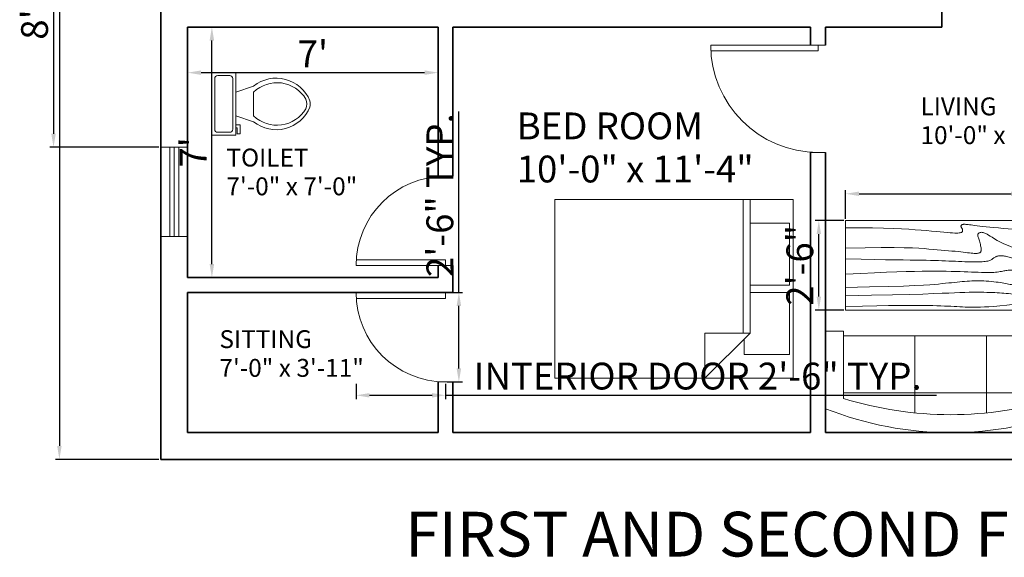
# Model space of a CAD drawing. Units: inches. Extents: x 3087 to 8148, y 1377 to 3709.
# Tile 1 of 6: x 3112 to 3443, y 1381 to 1561. Entities that reach past the tile are written whole.
import ezdxf

# ---------------------------------------------------------------- set-up
doc = ezdxf.new("R2010")
doc.units = ezdxf.units.IN
for name, color, linetype, lineweight, true_color in [('A-ANNO-DIMS', 244, 'Continuous', 18, 0x991b1e), ('A-ANNO-TEXT', 244, 'Continuous', 25, 0x991b1e), ('A-AREA-IDEN', 244, 'Continuous', 18, 0x991b1e), ('A-DOOR', 146, 'Continuous', 18, 0x105689), ('A-GLAZ', 146, 'Continuous', 18, 0x105689), ('A-WALL', 241, 'Continuous', 35, 0xf7abae)]:
    doc.layers.add(name, color=color, linetype=linetype, lineweight=lineweight, true_color=true_color)
doc.layers.add('A-FLOR-FIXT', color=9, linetype='Continuous', lineweight=18)
doc.layers.add('A-FURN', color=8, linetype='Continuous', lineweight=18)
doc.styles.get("Standard").update_dxf_attribs({"font": 'arial.ttf'})
doc.dimstyles.new('ISO-25', dxfattribs={"dimtxt": 9, "dimasz": 4.5, "dimexe": 1.25, "dimexo": 0.625, "dimtad": 1, "dimdec": 0, "dimlunit": 3, "dimtxsty": 'Standard', "dimcen": 2.5, "dimadec": 0, "dimazin": 0, "dimtfac": 1, "dimtdec": 0, "dimtmove": 0, "dimatfit": 3, "dimfxl": 1, "dimarcsym": 0})

# ---------------------------------------------------------------- blocks, each defined once
blk = doc.blocks.new('Bed - Queen')
for p, q in [((0, -80.00003), (0, 0)), ((0, 0), (59.99999, 0)), ((59.99999, 0), (59.99999, -80.00003)), ((7.99999, -1.2), (28.79998, -1.2)), ((7.99999, -14.4), (7.99999, -1.2)), ((28.79998, -1.2), (28.79998, -14.4)), ((31.19999, -1.2), (51.99999, -1.2)), ((31.19999, -14.4), (31.19999, -1.2)), ((51.99999, -1.2), (51.99999, -16.4)), ((0, -14.4), (44.8, -14.4)), ((59.99999, -29.6), (44.8, -14.4)), ((44.8, -14.4), (44.8, -29.6)), ((51.99999, -16.4), (46.79936, -16.4)), ((44.8, -16.8), (0, -16.8)), ((44.8, -29.6), (59.99999, -29.6)), ((59.99999, -80.00003), (0, -80.00003))]:
    blk.add_line(p, q)
blk = doc.blocks.new('Table - Rectangular Woodgrain 60 x 30 in.')
for p, q in [((0, 0), (0, -30)), ((60, 0), (0, 0)), ((60, -30), (60, 0)), ((0, -30), (60, -30))]:
    blk.add_line(p, q)
for points in [[(0, -2.4), (4.8155, -2.418), (9.0302, -2.4688), (12.709, -2.5477), (15.9167, -2.65), (18.7181, -2.7711), (21.1781, -2.9063), (23.3616, -3.0508), (25.3333, -3.2), (27.1477, -3.3495), (28.8172, -3.4958), (30.3437, -3.636), (31.7291, -3.7667), (32.9756, -3.8849), (34.0849, -3.9875), (35.059, -4.0714), (35.9, -4.1334), (36.6114, -4.1711), (37.2041, -4.1854), (37.6906, -4.1779), (38.0833, -4.15), (38.3948, -4.1034), (38.6375, -4.0396), (38.8239, -3.9602), (38.9666, -3.8667), (39.0764, -3.7608), (39.1573, -3.6448), (39.2116, -3.521), (39.2416, -3.3917), (39.2498, -3.2593), (39.2385, -3.1261), (39.21, -2.9944), (39.1666, -2.8667), (39.111, -2.7447), (39.0468, -2.6281), (38.978, -2.5163), (38.9083, -2.4083), (38.8418, -2.3035), (38.7823, -2.201), (38.7337, -2.1001), (38.7, -2), (38.6844, -1.9003), (38.6875, -1.8021), (38.7094, -1.707), (38.75, -1.6167), (38.8094, -1.5326), (38.8875, -1.4563), (38.9844, -1.3893), (39.1, -1.3333), (39.2351, -1.2896), (39.3937, -1.2583), (39.5804, -1.2396), (39.8, -1.2333), (40.057, -1.2396), (40.3562, -1.2583), (40.7023, -1.2896), (41.1, -1.3333), (41.5547, -1.3895), (42.0755, -1.4573), (42.6721, -1.5361), (43.3542, -1.625), (44.1316, -1.7233), (45.014, -1.8302), (46.0114, -1.9449), (47.1333, -2.0667), (48.3862, -2.1947), (49.7625, -2.3281), (51.2513, -2.4663), (52.8416, -2.6083), (54.5226, -2.7535), (56.2833, -2.9011), (58.1127, -3.0501), (60, -3.2)], [(0, -9.2), (6.5759, -9.0858), (11.9385, -9.0365), (16.2527, -9.0418), (19.6833, -9.0917), (22.3952, -9.1759), (24.5531, -9.2844), (26.322, -9.4069), (27.8666, -9.5333), (29.3241, -9.6553), (30.7203, -9.7719), (32.0532, -9.8837), (33.3208, -9.9917), (34.5213, -10.0965), (35.6526, -10.199), (36.7128, -10.2999), (37.7, -10.4), (38.6129, -10.4996), (39.4531, -10.5969), (40.223, -10.6895), (40.925, -10.775), (41.5613, -10.8512), (42.1344, -10.9156), (42.6465, -10.966), (43.1, -11), (43.4976, -11.0158), (43.8437, -11.0136), (44.143, -10.9942), (44.4, -10.9583), (44.6195, -10.9069), (44.8062, -10.8406), (44.9648, -10.7603), (45.1, -10.6667), (45.2155, -10.5598), (45.3114, -10.4365), (45.3871, -10.2929), (45.4416, -10.125), (45.4743, -9.929), (45.4844, -9.7011), (45.4709, -9.4371), (45.4333, -9.1333), (45.3716, -8.7883), (45.2896, -8.4104), (45.1919, -8.0107), (45.0833, -7.6), (44.9685, -7.1893), (44.8521, -6.7896), (44.7388, -6.4117), (44.6333, -6.0667), (44.54, -5.7628), (44.4614, -5.4979), (44.4001, -5.2675), (44.3583, -5.0667), (44.3384, -4.8909), (44.3427, -4.7354), (44.3736, -4.5956), (44.4333, -4.4667), (44.5236, -4.3453), (44.6427, -4.2333), (44.7884, -4.1339), (44.9583, -4.05), (45.1501, -3.9849), (45.3614, -3.9417), (45.59, -3.9234), (45.8333, -3.9333), (46.0915, -3.9749), (46.3734, -4.0531), (46.6906, -4.1736), (47.0542, -4.3417), (47.4756, -4.5629), (47.9661, -4.8427), (48.5372, -5.1866), (49.2, -5.6), (49.9676, -6.0844), (50.8594, -6.625), (51.8965, -7.2031), (53.1, -7.8), (54.491, -8.3969), (56.0906, -8.975), (57.9199, -9.5156), (60, -10)], [(0, -12.8), (5.1847, -12.9322), (9.6213, -13.0323), (13.3963, -13.1059), (16.5958, -13.1583), (19.3063, -13.1952), (21.614, -13.2219), (23.6054, -13.2439), (25.3666, -13.2667), (26.9728, -13.2947), (28.4531, -13.3281), (29.8256, -13.3663), (31.1083, -13.4083), (32.3191, -13.4535), (33.476, -13.501), (34.597, -13.5501), (35.7, -13.6), (36.7984, -13.6497), (37.8875, -13.6979), (38.9578, -13.743), (40, -13.7833), (41.0047, -13.8174), (41.9625, -13.8438), (42.864, -13.8607), (43.7, -13.8667), (44.4631, -13.8604), (45.1552, -13.8417), (45.7801, -13.8104), (46.3416, -13.7667), (46.8439, -13.7104), (47.2906, -13.6417), (47.6858, -13.5604), (48.0333, -13.4667), (48.3375, -13.3608), (48.6042, -13.2448), (48.8396, -13.121), (49.05, -12.9917), (49.2417, -12.8593), (49.4208, -12.7261), (49.5937, -12.5944), (49.7667, -12.4667), (49.9452, -12.3451), (50.1323, -12.2313), (50.3303, -12.1268), (50.5416, -12.0333), (50.7686, -11.9524), (51.0135, -11.8854), (51.2788, -11.8341), (51.5666, -11.8), (51.8785, -11.7843), (52.2116, -11.7865), (52.562, -11.8059), (52.926, -11.8417), (53.2998, -11.8931), (53.6795, -11.9594), (54.0614, -12.0397), (54.4416, -12.1333), (54.8223, -12.2401), (55.2293, -12.3625), (55.6942, -12.5037), (56.2489, -12.6667), (56.9251, -12.8547), (57.7545, -13.0708), (58.7689, -13.3182), (60, -13.6)], [(0, -18), (5.124, -17.7273), (9.6609, -17.5057), (13.6705, -17.3303), (17.2125, -17.1958), (20.3467, -17.0973), (23.1328, -17.0297), (25.6307, -16.9878), (27.9, -16.9667), (29.9928, -16.9617), (31.9302, -16.9703), (33.7254, -16.9907), (35.3917, -17.0208), (36.9423, -17.0588), (38.3906, -17.1026), (39.7499, -17.1503), (41.0333, -17.2), (42.2519, -17.2496), (43.4073, -17.2969), (44.4986, -17.3395), (45.525, -17.375), (46.4858, -17.4012), (47.3802, -17.4156), (48.2074, -17.416), (48.9667, -17.4), (49.6583, -17.3662), (50.2872, -17.3167), (50.8595, -17.2547), (51.3812, -17.1833), (51.8584, -17.1057), (52.2971, -17.025), (52.7034, -16.9443), (53.0833, -16.8667), (53.443, -16.7951), (53.789, -16.7313), (54.128, -16.6768), (54.4666, -16.6334), (54.8115, -16.6024), (55.1693, -16.5854), (55.5465, -16.5841), (55.95, -16.6), (56.3828, -16.6337), (56.8346, -16.6823), (57.2915, -16.7418), (57.7396, -16.8084), (58.165, -16.878), (58.5539, -16.9469), (58.8924, -17.0111), (59.1666, -17.0667), (59.3679, -17.1107), (59.5078, -17.1438), (59.6032, -17.1675), (59.6708, -17.1833), (59.7275, -17.193), (59.7901, -17.1979), (59.8753, -17.1998), (60, -17.2)], [(0, -22.4), (8.0098, -22.2501), (14.4094, -22.1011), (19.4168, -21.9535), (23.25, -21.8083), (26.1269, -21.6663), (28.2656, -21.5281), (29.884, -21.3947), (31.2, -21.2667), (32.3967, -21.1448), (33.5172, -21.0292), (34.5697, -20.9198), (35.5625, -20.8167), (36.5037, -20.7198), (37.4015, -20.6292), (38.2642, -20.5448), (39.1, -20.4667), (39.9164, -20.3951), (40.7187, -20.3313), (41.5117, -20.2768), (42.3, -20.2333), (43.0883, -20.2024), (43.8812, -20.1854), (44.6836, -20.1841), (45.5, -20.2), (46.3328, -20.234), (47.1747, -20.2844), (48.0163, -20.3488), (48.8479, -20.425), (49.66, -20.5106), (50.4429, -20.6031), (51.1872, -20.7004), (51.8833, -20.8), (52.5246, -20.8999), (53.1166, -20.9995), (53.6681, -21.0983), (54.1875, -21.1958), (54.6834, -21.2919), (55.1646, -21.3859), (55.6394, -21.4777), (56.1167, -21.5667), (56.6028, -21.6515), (57.0961, -21.7266), (57.5929, -21.7852), (58.0896, -21.8208), (58.5823, -21.8268), (59.0674, -21.7964), (59.5412, -21.723), (60, -21.6)], [(0, -25.2), (8.6355, -25.0504), (15.7026, -24.9031), (21.4049, -24.7606), (25.9458, -24.625), (29.529, -24.4988), (32.3578, -24.3844), (34.6359, -24.284), (36.5667, -24.2), (38.3213, -24.1341), (39.9417, -24.0854), (41.437, -24.0523), (42.8167, -24.0333), (44.0901, -24.0268), (45.2667, -24.0313), (46.3557, -24.0451), (47.3667, -24.0667), (48.309, -24.0947), (49.1928, -24.1287), (50.0284, -24.168), (50.826, -24.2125), (51.5959, -24.2617), (52.3483, -24.3151), (53.0935, -24.3725), (53.8417, -24.4334), (54.6009, -24.497), (55.3699, -24.561), (56.1454, -24.6226), (56.9239, -24.6792), (57.7021, -24.7279), (58.4764, -24.7662), (59.2435, -24.7911), (60, -24.8)], [(0, -28.8), (5.6867, -28.6681), (10.45, -28.5698), (14.407, -28.5012), (17.675, -28.4584), (20.3711, -28.4374), (22.6125, -28.4344), (24.5164, -28.4455), (26.2, -28.4667), (27.762, -28.4947), (29.2276, -28.5281), (30.6033, -28.5663), (31.8958, -28.6084), (33.1118, -28.6535), (34.2578, -28.7011), (35.3405, -28.7501), (36.3666, -28.8), (37.3443, -28.8497), (38.288, -28.8974), (39.2137, -28.9412), (40.1375, -28.9792), (41.0753, -29.0093), (42.0432, -29.0297), (43.0572, -29.0384), (44.1333, -29.0333), (45.2936, -29.0114), (46.5843, -28.9641), (48.0579, -28.8816), (49.7666, -28.7542), (51.7629, -28.5721), (54.0989, -28.3255), (56.8272, -28.0048), (60, -27.6)]]:
    blk.add_lwpolyline(points)
blk = doc.blocks.new('Toilet - top')
for p, q in [((9.5, -6), (9.5, -2)), ((-10, -8.5), (-8, -8.5)), ((-10, -9.5), (-10, -8.5)), ((-7, -9.5), (-10, -9.5)), ((-8, -8.5), (-8, -8)), ((-7, -8), (-7, -9.5)), ((-4, -8), (-6, -14)), ((4, -8), (6, -14)), ((4, -14), (-4, -14))]:
    blk.add_line(p, q)
blk.add_lwpolyline([(10.5, -8), (10.5, 0), (-10.5, 0), (-10.5, -8)], close=True)
for points in [[(-9.5, -2), (-9.5, -6)], [(8.5, -1), (-8.5, -1)], [(-8.5, -7), (8.5, -7)]]:
    blk.add_lwpolyline(points)
for centre, radius, start, end in [((-8.62, -1.88), 0.884, 81.8699, 188.1301), ((8.62, -1.88), 0.884, 351.8699, 98.1301), ((-8.62, -6.12), 0.884, 171.8699, 278.1301), ((8.62, -6.12), 0.884, 261.8699, 8.1301), ((3.52, -21.58), 12.17, 141.4691, 247.9714), ((4.2, -21.82), 11.33, 136.3677, 238.9468), ((-3.52, -21.58), 12.17, 292.0284, 38.5307), ((-4.2, -21.82), 11.33, 301.053, 43.6321), ((0, -27.88), 4, 245.7318, 294.2682), ((0, -29), 4, 254.8605, 285.1395)]:
    blk.add_arc(centre, radius, start, end)
blk = doc.blocks.new('Sofa - Roundback 7 ft.')
for p, q in [((-12.00002, -32.4421), (-12.00003, -6.5971)), ((11.99997, -32.4421), (11.99998, -6.5971)), ((-36.000027, -34), (-36.000027, -11.4696)), ((35.99998, -34), (35.99998, -11.4696)), ((-35.999844, -13.3819), (35.9998, -13.3819)), ((-36.000027, -32.4421), (35.99998, -32.4421))]:
    blk.add_line(p, q)
for points in [[(-36.000027, -34), (-42.000027, -34), (-42.000027, -8)], [(41.99998, -8), (41.99998, -34), (35.99998, -34)]]:
    blk.add_lwpolyline(points)
for centre, radius, start, end in [((0, -114.25), 114.25, 68.43141, 111.5686), ((-0.00001, -127.1968), 121.1968, 72.72033, 107.2797)]:
    blk.add_arc(centre, radius, start, end)
blk = doc.blocks.new('*D15')
at = {"layer": 'A-ANNO-DIMS', "color": 0, "lineweight": -2, "transparency": 16777216}
for p, q in [((3210.19, 1558.96), (3175.7, 1558.96)), ((3176.95, 1479.46), (3176.95, 1554.46)), ((3201.15, 1474.96), (3175.7, 1474.96))]:
    blk.add_line(p, q, dxfattribs=at)
at = {"layer": 'A-ANNO-DIMS', "color": 0, "transparency": 16777216}
for points in [[(3176.2, 1554.46), (3177.7, 1554.46), (3176.95, 1558.96)], [(3176.2, 1479.46), (3177.7, 1479.46), (3176.95, 1474.96)]]:
    blk.add_solid(points, dxfattribs=at)
at = {"layer": 'Defpoints', "color": 0, "transparency": 16777216}
for p in [(3176.95, 1558.96), (3210.82, 1558.96), (3201.77, 1474.96)]:
    blk.add_point(p, dxfattribs=at)
at = {"layer": 'A-ANNO-DIMS', "color": 0, "transparency": 16777216, "insert": (3171.82, 1516.96), "char_height": 9, "attachment_point": 5, "rotation": 90}
blk.add_mtext("7'", dxfattribs=at)
blk = doc.blocks.new('*D16')
at = {"layer": 'A-ANNO-DIMS', "color": 0, "lineweight": -2, "transparency": 16777216}
for p, q in [((3168.82, 1544.33), (3168.82, 1544.95)), ((3173.32, 1543.7), (3248.32, 1543.7)), ((3252.82, 1544.33), (3252.82, 1544.95))]:
    blk.add_line(p, q, dxfattribs=at)
at = {"layer": 'A-ANNO-DIMS', "color": 0, "transparency": 16777216}
for points in [[(3173.32, 1544.45), (3173.32, 1542.95), (3168.82, 1543.7)], [(3248.32, 1544.45), (3248.32, 1542.95), (3252.82, 1543.7)]]:
    blk.add_solid(points, dxfattribs=at)
at = {"layer": 'Defpoints', "color": 0, "transparency": 16777216}
for p in [(3168.82, 1543.7), (3252.82, 1543.7), (3252.82, 1543.7)]:
    blk.add_point(p, dxfattribs=at)
at = {"layer": 'A-ANNO-DIMS', "color": 0, "transparency": 16777216, "insert": (3210.82, 1548.83), "char_height": 9, "attachment_point": 5}
blk.add_mtext("7'", dxfattribs=at)
blk = doc.blocks.new('*D18')
at = {"layer": 'A-ANNO-DIMS', "color": 0, "lineweight": -2, "transparency": 16777216}
for p, q in [((3159.19, 2073.96), (3124.53, 2073.96)), ((3125.78, 2069.46), (3125.78, 1418.46)), ((3159.19, 1413.96), (3124.53, 1413.96))]:
    blk.add_line(p, q, dxfattribs=at)
at = {"layer": 'A-ANNO-DIMS', "color": 0, "transparency": 16777216}
for points in [[(3125.03, 2069.46), (3126.53, 2069.46), (3125.78, 2073.96)], [(3125.03, 1418.46), (3126.53, 1418.46), (3125.78, 1413.96)]]:
    blk.add_solid(points, dxfattribs=at)
at = {"layer": 'Defpoints', "color": 0, "transparency": 16777216}
for p in [(3159.82, 2073.96), (3125.78, 1413.96), (3159.82, 1413.96)]:
    blk.add_point(p, dxfattribs=at)
at = {"layer": 'A-ANNO-DIMS', "color": 0, "transparency": 16777216, "insert": (3120.58, 1743.96), "char_height": 9, "attachment_point": 5, "rotation": 90}
blk.add_mtext("55'", dxfattribs=at)
blk = doc.blocks.new('DOOR-SINGLE-30IN')
for p, q in [((0, 30), (30, 30)), ((30, 30), (30, 28)), ((0, 28), (30, 28))]:
    blk.add_line(p, q)
blk.add_arc((30, 30), 30, 180, 270)
blk = doc.blocks.new('DOOR-SINGLE-36IN')
for p, q in [((0, 2), (36, 2)), ((36, 0), (36, 2)), ((0, 0), (36, 0))]:
    blk.add_line(p, q)
blk.add_arc((36, 0), 36, 90, 180)
blk = doc.blocks.new('WINDOW-30IN')
for p, q in [((0, 0), (0, 30)), ((9, 30), (0, 30)), ((3, 30), (3, 0)), ((4.5, 30), (4.5, 0)), ((6, 30), (6, 0)), ((9, 30), (9, 0)), ((9, 0), (0, 0))]:
    blk.add_line(p, q)
blk = doc.blocks.new('*D27')
at = {"layer": 'A-ANNO-DIMS', "color": 0, "lineweight": -2, "transparency": 16777216}
for p, q in [((3225.32, 1439.34), (3225.32, 1434.21)), ((3255.32, 1439.34), (3255.32, 1434.21)), ((3229.82, 1435.46), (3250.82, 1435.46)), ((3255.32, 1435.46), (3420.05, 1435.46))]:
    blk.add_line(p, q, dxfattribs=at)
at = {"layer": 'A-ANNO-DIMS', "color": 0, "transparency": 16777216}
for points in [[(3229.82, 1436.21), (3229.82, 1434.71), (3225.32, 1435.46)], [(3250.82, 1436.21), (3250.82, 1434.71), (3255.32, 1435.46)]]:
    blk.add_solid(points, dxfattribs=at)
at = {"layer": 'Defpoints', "color": 0, "transparency": 16777216}
for p in [(3225.32, 1439.96), (3255.32, 1439.96), (3255.32, 1435.46)]:
    blk.add_point(p, dxfattribs=at)
at = {"layer": 'A-ANNO-DIMS', "color": 0, "transparency": 16777216, "insert": (3339.94, 1440.74), "char_height": 9, "attachment_point": 5}
blk.add_mtext('INTERIOR DOOR 2\'-6" TYP.', dxfattribs=at)
blk = doc.blocks.new('*D28')
at = {"layer": 'A-ANNO-DIMS', "color": 0, "lineweight": -2, "transparency": 16777216}
for p, q in [((3259.82, 1469.96), (3259.82, 1530.72)), ((3255.94, 1469.96), (3261.07, 1469.96)), ((3259.82, 1444.46), (3259.82, 1465.46)), ((3255.94, 1439.96), (3261.07, 1439.96))]:
    blk.add_line(p, q, dxfattribs=at)
at = {"layer": 'A-ANNO-DIMS', "color": 0, "transparency": 16777216}
for points in [[(3259.07, 1465.46), (3260.57, 1465.46), (3259.82, 1469.96)], [(3259.07, 1444.46), (3260.57, 1444.46), (3259.82, 1439.96)]]:
    blk.add_solid(points, dxfattribs=at)
at = {"layer": 'Defpoints', "color": 0, "transparency": 16777216}
for p in [(3255.32, 1469.96), (3259.82, 1469.96), (3255.32, 1439.96)]:
    blk.add_point(p, dxfattribs=at)
at = {"layer": 'A-ANNO-DIMS', "color": 0, "transparency": 16777216, "insert": (3254.6, 1502.59), "char_height": 9, "attachment_point": 5, "rotation": 90}
blk.add_mtext('2\'-6" TYP.', dxfattribs=at)
blk = doc.blocks.new('*D51')
at = {"layer": 'A-ANNO-DIMS', "color": 0, "lineweight": -2, "transparency": 16777216}
for p, q in [((3389.59, 1494.68), (3389.59, 1504.31)), ((3449.59, 1494.68), (3449.59, 1504.31)), ((3394.09, 1503.06), (3445.09, 1503.06)), ((3449.59, 1503.06), (3522.82, 1503.06))]:
    blk.add_line(p, q, dxfattribs=at)
at = {"layer": 'A-ANNO-DIMS', "color": 0, "transparency": 16777216}
for points in [[(3394.09, 1503.81), (3394.09, 1502.31), (3389.59, 1503.06)], [(3445.09, 1503.81), (3445.09, 1502.31), (3449.59, 1503.06)]]:
    blk.add_solid(points, dxfattribs=at)
at = {"layer": 'Defpoints', "color": 0, "transparency": 16777216}
for p in [(3449.59, 1503.06), (3389.59, 1494.06), (3449.59, 1494.06)]:
    blk.add_point(p, dxfattribs=at)
at = {"layer": 'A-ANNO-DIMS', "color": 0, "transparency": 16777216, "insert": (3488.45, 1508.28), "char_height": 9, "attachment_point": 5}
blk.add_mtext('TABLE 5\'-0"', dxfattribs=at)
blk = doc.blocks.new('*D52')
at = {"layer": 'A-ANNO-DIMS', "color": 0, "lineweight": -2, "transparency": 16777216}
for p, q in [((3388.97, 1494.06), (3379.34, 1494.06)), ((3380.59, 1468.56), (3380.59, 1489.56)), ((3388.97, 1464.06), (3379.34, 1464.06))]:
    blk.add_line(p, q, dxfattribs=at)
at = {"layer": 'A-ANNO-DIMS', "color": 0, "transparency": 16777216}
for points in [[(3379.84, 1489.56), (3381.34, 1489.56), (3380.59, 1494.06)], [(3379.84, 1468.56), (3381.34, 1468.56), (3380.59, 1464.06)]]:
    blk.add_solid(points, dxfattribs=at)
at = {"layer": 'Defpoints', "color": 0, "transparency": 16777216}
for p in [(3380.59, 1494.06), (3389.59, 1494.06), (3389.59, 1464.06)]:
    blk.add_point(p, dxfattribs=at)
at = {"layer": 'A-ANNO-DIMS', "color": 0, "transparency": 16777216, "insert": (3375.37, 1479.06), "char_height": 9, "attachment_point": 5, "rotation": 90}
blk.add_mtext('2\'-6"', dxfattribs=at)
blk = doc.blocks.new('*D64')
at = {"layer": 'A-ANNO-DIMS', "color": 0, "lineweight": -2, "transparency": 16777216}
for p, q in [((3159.19, 1624.74), (3122.57, 1624.74)), ((3123.82, 1620.24), (3123.82, 1523.18)), ((3159.19, 1518.68), (3122.57, 1518.68))]:
    blk.add_line(p, q, dxfattribs=at)
at = {"layer": 'A-ANNO-DIMS', "color": 0, "transparency": 16777216}
for points in [[(3123.07, 1620.24), (3124.57, 1620.24), (3123.82, 1624.74)], [(3123.07, 1523.18), (3124.57, 1523.18), (3123.82, 1518.68)]]:
    blk.add_solid(points, dxfattribs=at)
at = {"layer": 'Defpoints', "color": 0, "transparency": 16777216}
for p in [(3159.82, 1624.74), (3123.82, 1518.68), (3159.82, 1518.68)]:
    blk.add_point(p, dxfattribs=at)
at = {"layer": 'A-ANNO-DIMS', "color": 0, "transparency": 16777216, "insert": (3118.6, 1571.71), "char_height": 9, "attachment_point": 5, "rotation": 90}
blk.add_mtext('8\'-10"', dxfattribs=at)

msp = doc.modelspace()

# ---------------------------------------------------------------- linework, layer by layer
at = {"layer": 'A-DOOR'}
for p, q in [((3377.82, 1552.96), (3382.82, 1552.96)), ((3377.82, 1516.96), (3382.82, 1516.96)), ((3252.82, 1508.96), (3257.82, 1508.96)), ((3252.82, 1478.96), (3257.82, 1478.96)), ((3252.82, 1439.96), (3257.82, 1439.96))]:
    msp.add_line(p, q, dxfattribs=at)
at = {"layer": 'A-WALL'}
for p, q in [((3159.82, 1413.96), (3159.82, 2073.96)), ((3421.82, 1558.96), (3421.82, 1563.96)), ((3168.82, 1558.96), (3252.82, 1558.96)), ((3168.82, 1474.96), (3168.82, 1558.96)), ((3252.82, 1508.96), (3252.82, 1558.96)), ((3257.82, 1508.96), (3257.82, 1558.96)), ((3257.82, 1558.96), (3377.82, 1558.96)), ((3377.82, 1552.96), (3377.82, 1558.96)), ((3382.82, 1552.96), (3382.82, 1558.96)), ((3382.82, 1558.96), (3421.82, 1558.96)), ((3377.82, 1422.96), (3377.82, 1516.96)), ((3382.82, 1422.96), (3382.82, 1516.96)), ((3252.82, 1474.96), (3252.82, 1478.96)), ((3257.82, 1469.96), (3257.82, 1478.96)), ((3168.82, 1474.96), (3252.82, 1474.96)), ((3168.82, 1422.96), (3168.82, 1469.96)), ((3168.82, 1469.96), (3257.82, 1469.96)), ((3252.82, 1422.96), (3252.82, 1439.96)), ((3257.82, 1422.96), (3257.82, 1439.96)), ((3252.82, 1422.96), (3168.82, 1422.96)), ((3377.82, 1422.96), (3257.82, 1422.96)), ((3502.82, 1422.96), (3382.82, 1422.96)), ((3639.82, 1413.96), (3159.82, 1413.96))]:
    msp.add_line(p, q, dxfattribs=at)

# ---------------------------------------------------------------- block references
at = {"layer": 'A-DOOR', "extrusion": (0, 0, -1), "zscale": -1, "rotation": 180}
for name, p in [('DOOR-SINGLE-36IN', (-3344.32, 1552.96)), ('DOOR-SINGLE-30IN', (-3225.32, 1508.96))]:
    msp.add_blockref(name, p, dxfattribs=at)
at = {"layer": 'A-DOOR'}
msp.add_blockref('DOOR-SINGLE-30IN', (3225.32, 1439.96), dxfattribs=at)
at = {"layer": 'A-FLOR-FIXT', "rotation": 90}
msp.add_blockref('Toilet - top', (3176.95, 1533.2), dxfattribs=at)
at = {"layer": 'A-FURN'}
for name, p, rotation in [('Bed - Queen', (3371.97, 1501.16), 270), ('Sofa - Roundback 7 ft.', (3424.82, 1422.96), 180)]:
    msp.add_blockref(name, p, dxfattribs=dict(at, rotation=rotation))
msp.add_blockref('Table - Rectangular Woodgrain 60 x 30 in.', (3389.59, 1494.06), dxfattribs=at)
at = {"layer": 'A-GLAZ'}
msp.add_blockref('WINDOW-30IN', (3159.82, 1488.68), dxfattribs=at)

# ---------------------------------------------------------------- texts
at = {"layer": 'A-ANNO-TEXT'}
msp.add_text('FIRST AND SECOND FLOOR ', height=15, dxfattribs=at).set_placement((3241.85, 1381.38))
at = {"layer": 'A-AREA-IDEN'}
for s, height, p in [('LIVING', 6, (3414.7, 1529.38)), ('BED ROOM ', 9, (3279.22, 1521.33)), ('10\'-0" x 11\'-4"', 6, (3414.7, 1519.74)), ('TOILET', 6, (3181.82, 1512.21)), ('10\'-0" x 11\'-4"', 9, (3279.22, 1506.87)), ('7\'-0" x 7\'-0"', 6, (3181.82, 1502.57)), ('SITTING', 6, (3179.48, 1451.3)), ('7\'-0" x 3\'-11"', 6, (3179.48, 1441.66))]:
    msp.add_text(s, height=height, dxfattribs=at).set_placement(p)

# ---------------------------------------------------------------- dimensions: what is measured, and where the dimension line sits
at = {"layer": 'A-ANNO-DIMS'}
for base, p1, p2, override, picture, middle in [((3125.78, 1413.96), (3159.82, 2073.96), (3159.82, 1413.96), {"dimclrd": 0, "dimclre": 0, "dimclrt": 0}, '*D18', (3120.58, 1743.96)), ((3123.82, 1518.68), (3159.82, 1624.74), (3159.82, 1518.68), {"dimdec": 1, "dimlfac": 1, "dimrnd": 0, "dimzin": 1, "dimdsep": 46, "dimlunit": 4, "dimfrac": 2}, '*D64', (3118.6, 1571.71)), ((3176.95, 1558.96), (3201.77, 1474.96), (3210.82, 1558.96), {"dimclrd": 0, "dimclre": 0, "dimclrt": 0}, '*D15', (3171.82, 1516.96)), ((3380.59, 1494.06), (3389.59, 1464.06), (3389.59, 1494.06), {"dimdec": 1, "dimlfac": 1, "dimrnd": 0, "dimzin": 1, "dimdsep": 46, "dimlunit": 4, "dimfrac": 2}, '*D52', (3375.37, 1479.06))]:
    dim = msp.add_linear_dim(base=base, p1=p1, p2=p2, angle=90, dimstyle='ISO-25', override=override, dxfattribs=at)
    dim.commit()
    dim.dimension.update_dxf_attribs({"geometry": picture, "text_midpoint": middle})
dim = msp.add_linear_dim(base=(3252.82, 1543.7), p1=(3168.82, 1543.7), p2=(3252.82, 1543.7), dimstyle='ISO-25', override={"dimclrd": 0, "dimclre": 0, "dimclrt": 0}, dxfattribs=at)
dim.commit()
dim.dimension.update_dxf_attribs({"geometry": '*D16', "text_midpoint": (3210.82, 1548.83)})
dim = msp.add_linear_dim(base=(3259.82, 1469.96), p1=(3255.32, 1439.96), p2=(3255.32, 1469.96), angle=90, text='<> TYP.', dimstyle='ISO-25', override={"dimdec": 1, "dimlfac": 1, "dimrnd": 0, "dimzin": 1, "dimdsep": 46, "dimlunit": 4, "dimfrac": 2}, dxfattribs=at)
dim.commit()
dim.dimension.update_dxf_attribs({"geometry": '*D28', "text_midpoint": (3254.6, 1502.59)})
for base, p1, p2, text, picture, middle in [((3449.59, 1503.06), (3389.59, 1494.06), (3449.59, 1494.06), 'TABLE <>', '*D51', (3488.45, 1508.28)), ((3255.32, 1435.46), (3225.32, 1439.96), (3255.32, 1439.96), 'INTERIOR DOOR <> TYP.', '*D27', (3339.94, 1440.74))]:
    dim = msp.add_linear_dim(base=base, p1=p1, p2=p2, text=text, dimstyle='ISO-25', override={"dimdec": 1, "dimlfac": 1, "dimrnd": 0, "dimzin": 1, "dimdsep": 46, "dimlunit": 4, "dimfrac": 2}, dxfattribs=at)
    dim.commit()
    dim.dimension.update_dxf_attribs({"geometry": picture, "text_midpoint": middle})

doc.saveas('drawing.dxf')
